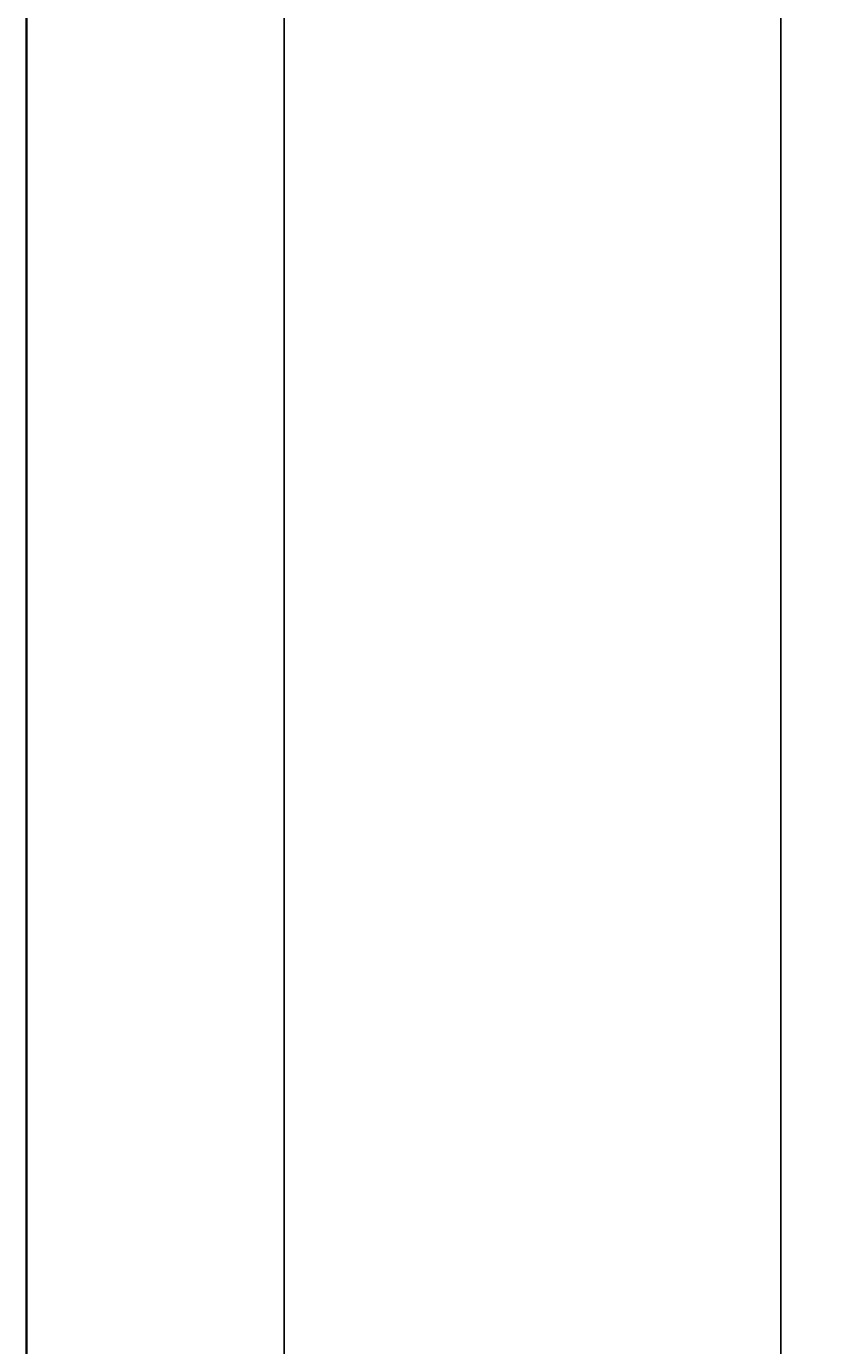
# Model space of a CAD drawing. Units: inches. Extents: x 1734 to 2405, y 1500 to 2491.
# Tile 3 of 14: x 1734 to 1797, y 1784 to 1888. Entities that reach past the tile are written whole.
import ezdxf

# ---------------------------------------------------------------- set-up
doc = ezdxf.new("R2010")
doc.units = ezdxf.units.IN
for name, color, linetype, lineweight in [('A-ANNO-DIMS', 2, 'Continuous', 18), ('A-ANNO-TTLB', 7, 'Continuous', 35), ('C-PROP', 7, 'Continuous', 25)]:
    doc.layers.add(name, color=color, linetype=linetype, lineweight=lineweight)
doc.styles.get("Standard").update_dxf_attribs({"font": 'arial.ttf'})
doc.dimstyles.get("Standard").update_dxf_attribs({"dimtxt": 0.18, "dimasz": 0.18, "dimexe": 0.18, "dimexo": 0.0625, "dimgap": 0.09, "dimtad": 0, "dimtih": 1, "dimtoh": 1, "dimdec": 4, "dimzin": 0, "dimdsep": 46, "dimtxsty": 'Standard', "dimcen": 0.09, "dimadec": 0, "dimazin": 0, "dimtfac": 1, "dimtdec": 4, "dimtofl": 0, "dimtmove": 0, "dimatfit": 3, "dimfxl": 1, "dimtolj": 1, "dimtzin": 0, "dimarcsym": 0})

# ---------------------------------------------------------------- blocks, each defined once
blk = doc.blocks.new('*D23')
at = {"layer": 'A-ANNO-DIMS', "color": 0, "lineweight": -2, "transparency": 16777216}
for p, q in [((1793.83, 2425.82), (1754.36, 2425.82)), ((1754.54, 2425.64), (1754.54, 2068.48)), ((1754.54, 1710.95), (1754.54, 2068.11)), ((1793.83, 1710.77), (1754.36, 1710.77))]:
    blk.add_line(p, q, dxfattribs=at)
at = {"layer": 'A-ANNO-DIMS', "color": 0, "transparency": 16777216}
for points in [[(1754.51, 2425.64), (1754.57, 2425.64), (1754.54, 2425.82)], [(1754.51, 1710.95), (1754.57, 1710.95), (1754.54, 1710.77)]]:
    blk.add_solid(points, dxfattribs=at)
at = {"layer": 'Defpoints', "color": 0, "transparency": 16777216}
for p in [(1754.54, 2425.82), (1793.89, 2425.82), (1793.89, 1710.77)]:
    blk.add_point(p, dxfattribs=at)
at = {"layer": 'A-ANNO-DIMS', "color": 0, "transparency": 16777216, "insert": (1754.54, 2068.3), "char_height": 0.18, "attachment_point": 5}
blk.add_mtext('\\A1;715', dxfattribs=at)

msp = doc.modelspace()

# ---------------------------------------------------------------- linework, layer by layer
at = {"layer": 'A-ANNO-TTLB'}
msp.add_lwpolyline([(1734.1307, 2491.1293), (2404.5589, 2491.1293), (2404.5589, 1500.293), (1734.1307, 1500.293)], close=True, dxfattribs=at)
at = {"layer": 'C-PROP'}
msp.add_line((1793.8942, 1891.8246), (1793.8942, 1710.7667), dxfattribs=at)

# ---------------------------------------------------------------- dimensions: what is measured, and where the dimension line sits
at = {"layer": 'A-ANNO-DIMS'}
dim = msp.add_linear_dim(base=(1754.5442, 2425.8246), p1=(1793.8942, 1710.7667), p2=(1793.8942, 2425.8246), angle=90, dimstyle='Standard', override={"dimdec": 0, "dimlfac": 1, "dimrnd": 0, "dimzin": 0, "dimdsep": 46, "dimlunit": 2}, dxfattribs=at)
dim.commit()
dim.dimension.update_dxf_attribs({"geometry": '*D23', "text_midpoint": (1754.5442, 2068.2956)})

doc.saveas('drawing.dxf')
